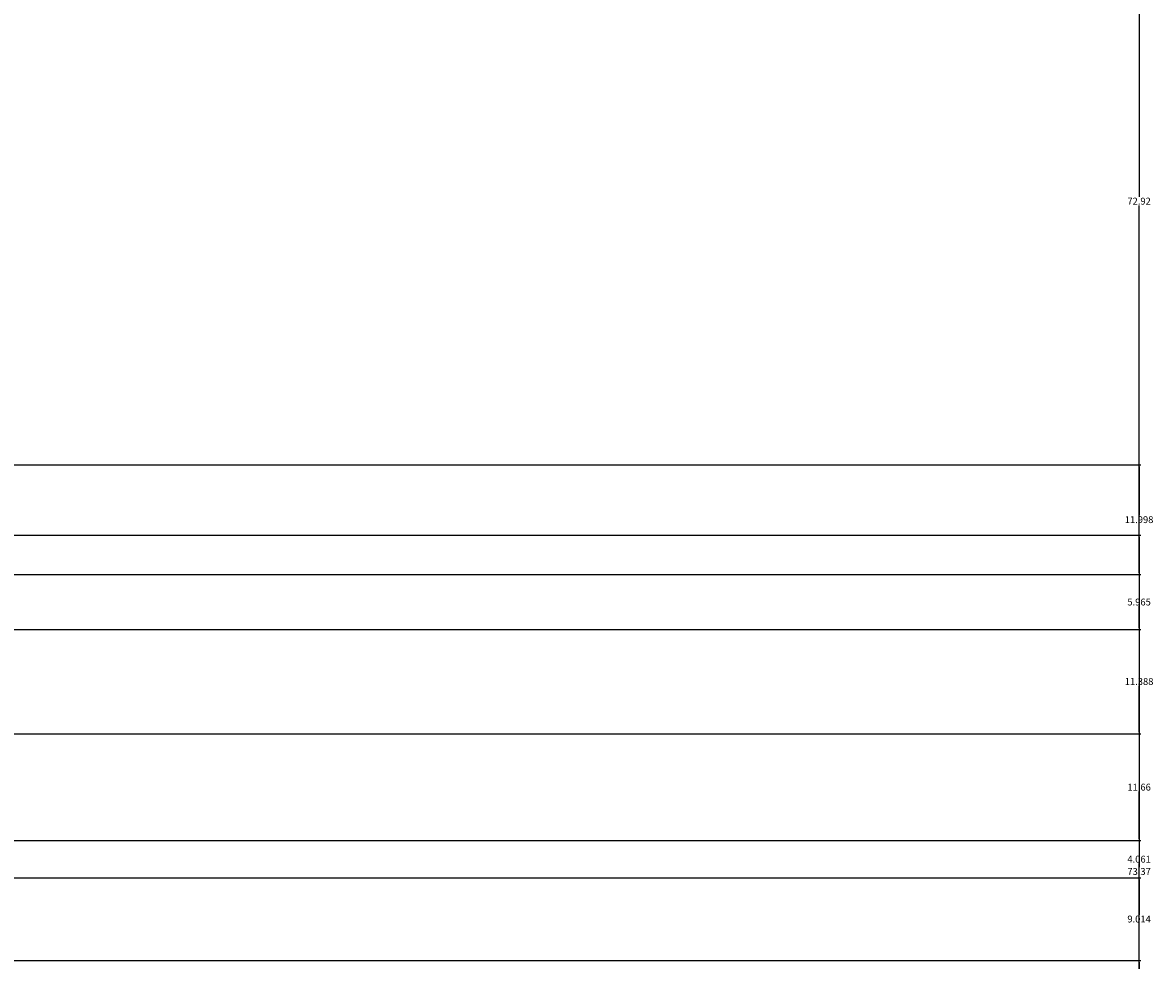
# Model space of a CAD drawing. Units: inches. Extents: x 62 to 566, y 66 to 528.
# Tile 19 of 20: x 443 to 566, y 298 to 401. Entities that reach past the tile are written whole.
import ezdxf

# ---------------------------------------------------------------- set-up
doc = ezdxf.new("R2010")
doc.units = ezdxf.units.IN
doc.header["$MEASUREMENT"] = 0
doc.layers.add('A-ANNO-DIMS', color=2, linetype='Continuous', lineweight=18)
doc.styles.get("Standard").update_dxf_attribs({"font": 'arial.ttf'})
doc.dimstyles.get("Standard").update_dxf_attribs({"dimtxt": 0.75, "dimasz": 0.18, "dimexe": 0.18, "dimexo": 0.0625, "dimgap": 0.09, "dimtad": 0, "dimtih": 1, "dimtoh": 1, "dimdec": 4, "dimzin": 0, "dimdsep": 46, "dimlunit": 4, "dimtxsty": 'Standard', "dimcen": 0.09, "dimadec": 0, "dimazin": 0, "dimtfac": 1, "dimtdec": 4, "dimtofl": 0, "dimtmove": 0, "dimatfit": 3, "dimfxl": 1, "dimtolj": 1, "dimtzin": 0, "dimarcsym": 0})

# ---------------------------------------------------------------- blocks, each defined once
blk = doc.blocks.new('*D23')
at = {"layer": 'A-ANNO-DIMS', "color": 0, "lineweight": -2, "transparency": 16777216}
for p, q in [((374.2, 344.78), (564.47, 344.78)), ((564.29, 344.6), (564.29, 308.57)), ((564.29, 271.59), (564.29, 307.62)), ((540.1, 271.41), (564.47, 271.41))]:
    blk.add_line(p, q, dxfattribs=at)
at = {"layer": 'A-ANNO-DIMS', "color": 0, "transparency": 16777216}
for points in [[(564.26, 344.6), (564.32, 344.6), (564.29, 344.78)], [(564.26, 271.59), (564.32, 271.59), (564.29, 271.41)]]:
    blk.add_solid(points, dxfattribs=at)
at = {"layer": 'Defpoints', "color": 0, "transparency": 16777216}
for p in [(374.14, 344.78), (564.29, 344.78), (540.04, 271.41)]:
    blk.add_point(p, dxfattribs=at)
at = {"layer": 'A-ANNO-DIMS', "color": 0, "transparency": 16777216, "insert": (564.29, 308.1), "char_height": 0.75, "attachment_point": 5}
blk.add_mtext('\\A1;73.37', dxfattribs=at)
blk = doc.blocks.new('*D24')
at = {"layer": 'A-ANNO-DIMS', "color": 0, "lineweight": -2, "transparency": 16777216}
for p, q in [((374.2, 417.71), (564.47, 417.71)), ((564.29, 417.53), (564.29, 381.72)), ((564.29, 344.96), (564.29, 380.77)), ((374.2, 344.78), (564.47, 344.78))]:
    blk.add_line(p, q, dxfattribs=at)
at = {"layer": 'A-ANNO-DIMS', "color": 0, "transparency": 16777216}
for points in [[(564.26, 417.53), (564.32, 417.53), (564.29, 417.71)], [(564.26, 344.96), (564.32, 344.96), (564.29, 344.78)]]:
    blk.add_solid(points, dxfattribs=at)
at = {"layer": 'Defpoints', "color": 0, "transparency": 16777216}
for p in [(374.14, 417.71), (564.29, 417.71), (374.14, 344.78)]:
    blk.add_point(p, dxfattribs=at)
at = {"layer": 'A-ANNO-DIMS', "color": 0, "transparency": 16777216, "insert": (564.29, 381.24), "char_height": 0.75, "attachment_point": 5}
blk.add_mtext('\\A1;72.92', dxfattribs=at)
blk = doc.blocks.new('*D91')
at = {"layer": 'A-ANNO-DIMS', "color": 0, "lineweight": -2, "transparency": 16777216}
for p, q in [((433.87, 298.4), (564.47, 298.4)), ((564.29, 298.22), (564.29, 297.15)), ((564.29, 295.13), (564.29, 296.2)), ((433.87, 294.95), (564.47, 294.95))]:
    blk.add_line(p, q, dxfattribs=at)
at = {"layer": 'A-ANNO-DIMS', "color": 0, "transparency": 16777216}
for points in [[(564.26, 298.22), (564.32, 298.22), (564.29, 298.4)], [(564.26, 295.13), (564.32, 295.13), (564.29, 294.95)]]:
    blk.add_solid(points, dxfattribs=at)
at = {"layer": 'Defpoints', "color": 0, "transparency": 16777216}
for p in [(433.81, 298.4), (564.29, 298.4), (433.81, 294.95)]:
    blk.add_point(p, dxfattribs=at)
at = {"layer": 'A-ANNO-DIMS', "color": 0, "transparency": 16777216, "insert": (564.29, 296.67), "char_height": 0.75, "attachment_point": 5}
blk.add_mtext('\\A1;3.449', dxfattribs=at)
blk = doc.blocks.new('*D92')
at = {"layer": 'A-ANNO-DIMS', "color": 0, "lineweight": -2, "transparency": 16777216}
for p, q in [((392.54, 307.41), (564.47, 307.41)), ((564.29, 307.23), (564.29, 303.38)), ((564.29, 298.58), (564.29, 302.43)), ((433.87, 298.4), (564.47, 298.4))]:
    blk.add_line(p, q, dxfattribs=at)
at = {"layer": 'A-ANNO-DIMS', "color": 0, "transparency": 16777216}
for points in [[(564.26, 307.23), (564.32, 307.23), (564.29, 307.41)], [(564.26, 298.58), (564.32, 298.58), (564.29, 298.4)]]:
    blk.add_solid(points, dxfattribs=at)
at = {"layer": 'Defpoints', "color": 0, "transparency": 16777216}
for p in [(392.48, 307.41), (564.29, 307.41), (433.81, 298.4)]:
    blk.add_point(p, dxfattribs=at)
at = {"layer": 'A-ANNO-DIMS', "color": 0, "transparency": 16777216, "insert": (564.29, 302.91), "char_height": 0.75, "attachment_point": 5}
blk.add_mtext('\\A1;9.014', dxfattribs=at)
blk = doc.blocks.new('*D93')
at = {"layer": 'A-ANNO-DIMS', "color": 0, "lineweight": -2, "transparency": 16777216}
for p, q in [((433.23, 311.47), (564.47, 311.47)), ((564.29, 311.29), (564.29, 309.92)), ((564.29, 307.59), (564.29, 308.97)), ((392.54, 307.41), (564.47, 307.41))]:
    blk.add_line(p, q, dxfattribs=at)
at = {"layer": 'A-ANNO-DIMS', "color": 0, "transparency": 16777216}
for points in [[(564.26, 311.29), (564.32, 311.29), (564.29, 311.47)], [(564.26, 307.59), (564.32, 307.59), (564.29, 307.41)]]:
    blk.add_solid(points, dxfattribs=at)
at = {"layer": 'Defpoints', "color": 0, "transparency": 16777216}
for p in [(433.16, 311.47), (564.29, 311.47), (392.48, 307.41)]:
    blk.add_point(p, dxfattribs=at)
at = {"layer": 'A-ANNO-DIMS', "color": 0, "transparency": 16777216, "insert": (564.29, 309.44), "char_height": 0.75, "attachment_point": 5}
blk.add_mtext('\\A1;4.061', dxfattribs=at)
blk = doc.blocks.new('*D94')
at = {"layer": 'A-ANNO-DIMS', "color": 0, "lineweight": -2, "transparency": 16777216}
for p, q in [((433.23, 323.13), (564.47, 323.13)), ((564.29, 322.95), (564.29, 317.78)), ((564.29, 311.65), (564.29, 316.83)), ((433.23, 311.47), (564.47, 311.47))]:
    blk.add_line(p, q, dxfattribs=at)
at = {"layer": 'A-ANNO-DIMS', "color": 0, "transparency": 16777216}
for points in [[(564.26, 322.95), (564.32, 322.95), (564.29, 323.13)], [(564.26, 311.65), (564.32, 311.65), (564.29, 311.47)]]:
    blk.add_solid(points, dxfattribs=at)
at = {"layer": 'Defpoints', "color": 0, "transparency": 16777216}
for p in [(433.16, 323.13), (564.29, 323.13), (433.16, 311.47)]:
    blk.add_point(p, dxfattribs=at)
at = {"layer": 'A-ANNO-DIMS', "color": 0, "transparency": 16777216, "insert": (564.29, 317.3), "char_height": 0.75, "attachment_point": 5}
blk.add_mtext('\\A1;11.66', dxfattribs=at)
blk = doc.blocks.new('*D95')
at = {"layer": 'A-ANNO-DIMS', "color": 0, "lineweight": -2, "transparency": 16777216}
for p, q in [((433.23, 334.52), (564.47, 334.52)), ((564.29, 334.34), (564.29, 329.3)), ((564.29, 323.31), (564.29, 328.35)), ((433.23, 323.13), (564.47, 323.13))]:
    blk.add_line(p, q, dxfattribs=at)
at = {"layer": 'A-ANNO-DIMS', "color": 0, "transparency": 16777216}
for points in [[(564.26, 334.34), (564.32, 334.34), (564.29, 334.52)], [(564.26, 323.31), (564.32, 323.31), (564.29, 323.13)]]:
    blk.add_solid(points, dxfattribs=at)
at = {"layer": 'Defpoints', "color": 0, "transparency": 16777216}
for p in [(433.16, 334.52), (564.29, 334.52), (433.16, 323.13)]:
    blk.add_point(p, dxfattribs=at)
at = {"layer": 'A-ANNO-DIMS', "color": 0, "transparency": 16777216, "insert": (564.29, 328.83), "char_height": 0.75, "attachment_point": 5}
blk.add_mtext('\\A1;11.388', dxfattribs=at)
blk = doc.blocks.new('*D96')
at = {"layer": 'A-ANNO-DIMS', "color": 0, "lineweight": -2, "transparency": 16777216}
for p, q in [((433.23, 340.49), (564.47, 340.49)), ((564.29, 340.31), (564.29, 337.98)), ((564.29, 334.7), (564.29, 337.03)), ((433.23, 334.52), (564.47, 334.52))]:
    blk.add_line(p, q, dxfattribs=at)
at = {"layer": 'A-ANNO-DIMS', "color": 0, "transparency": 16777216}
for points in [[(564.26, 340.31), (564.32, 340.31), (564.29, 340.49)], [(564.26, 334.7), (564.32, 334.7), (564.29, 334.52)]]:
    blk.add_solid(points, dxfattribs=at)
at = {"layer": 'Defpoints', "color": 0, "transparency": 16777216}
for p in [(433.16, 340.49), (564.29, 340.49), (433.16, 334.52)]:
    blk.add_point(p, dxfattribs=at)
at = {"layer": 'A-ANNO-DIMS', "color": 0, "transparency": 16777216, "insert": (564.29, 337.5), "char_height": 0.75, "attachment_point": 5}
blk.add_mtext('\\A1;5.965', dxfattribs=at)
blk = doc.blocks.new('*D97')
at = {"layer": 'A-ANNO-DIMS', "color": 0, "lineweight": -2, "transparency": 16777216}
for p, q in [((439.75, 352.48), (564.47, 352.48)), ((564.29, 352.3), (564.29, 346.96)), ((564.29, 340.67), (564.29, 346.01)), ((433.23, 340.49), (564.47, 340.49))]:
    blk.add_line(p, q, dxfattribs=at)
at = {"layer": 'A-ANNO-DIMS', "color": 0, "transparency": 16777216}
for points in [[(564.26, 352.3), (564.32, 352.3), (564.29, 352.48)], [(564.26, 340.67), (564.32, 340.67), (564.29, 340.49)]]:
    blk.add_solid(points, dxfattribs=at)
at = {"layer": 'Defpoints', "color": 0, "transparency": 16777216}
for p in [(439.69, 352.48), (564.29, 352.48), (433.16, 340.49)]:
    blk.add_point(p, dxfattribs=at)
at = {"layer": 'A-ANNO-DIMS', "color": 0, "transparency": 16777216, "insert": (564.29, 346.49), "char_height": 0.75, "attachment_point": 5}
blk.add_mtext('\\A1;11.998', dxfattribs=at)

msp = doc.modelspace()

# ---------------------------------------------------------------- dimensions: what is measured, and where the dimension line sits
at = {"layer": 'A-ANNO-DIMS'}
for base, p1, p2, override, picture, middle in [((564.2868, 417.7059), (374.1373, 344.7821), (374.1373, 417.7059), {"dimdec": 2, "dimlfac": 1, "dimrnd": 0, "dimzin": 0, "dimdsep": 46, "dimlunit": 2}, '*D24', (564.2868, 381.244)), ((564.28678, 352.4848), (433.16362, 340.48631), (439.68784, 352.4848), {"dimdec": 3, "dimlfac": 1, "dimrnd": 0, "dimzin": 0, "dimdsep": 46, "dimlunit": 2}, '*D97', (564.28678, 346.48556)), ((564.2868, 344.7821), (540.0368, 271.4128), (374.1373, 344.7821), {"dimdec": 2, "dimlfac": 1, "dimrnd": 0, "dimzin": 0, "dimdsep": 46, "dimlunit": 2}, '*D23', (564.2868, 308.0974)), ((564.2868, 340.4863), (433.1636, 334.5211), (433.1636, 340.4863), {"dimdec": 3, "dimlfac": 1, "dimrnd": 0, "dimzin": 0, "dimdsep": 46, "dimlunit": 2}, '*D96', (564.2868, 337.5037)), ((564.2868, 334.5211), (433.1636, 323.1329), (433.1636, 334.5211), {"dimdec": 3, "dimlfac": 1, "dimrnd": 0, "dimzin": 0, "dimdsep": 46, "dimlunit": 2}, '*D95', (564.2868, 328.827)), ((564.2868, 323.1329), (433.1636, 311.4736), (433.1636, 323.1329), {"dimdec": 2, "dimlfac": 1, "dimrnd": 0, "dimzin": 0, "dimdsep": 46, "dimlunit": 2}, '*D94', (564.2868, 317.3033)), ((564.2868, 311.4736), (392.4793, 307.4128), (433.1636, 311.4736), {"dimdec": 3, "dimlfac": 1, "dimrnd": 0, "dimzin": 0, "dimdsep": 46, "dimlunit": 2}, '*D93', (564.2868, 309.4432)), ((564.2868, 307.4128), (433.8102, 298.3985), (392.4793, 307.4128), {"dimdec": 3, "dimlfac": 1, "dimrnd": 0, "dimzin": 0, "dimdsep": 46, "dimlunit": 2}, '*D92', (564.2868, 302.9056)), ((564.2868, 298.3985), (433.8102, 294.9497), (433.8102, 298.3985), {"dimdec": 3, "dimlfac": 1, "dimrnd": 0, "dimzin": 0, "dimdsep": 46, "dimlunit": 2}, '*D91', (564.2868, 296.6741))]:
    dim = msp.add_linear_dim(base=base, p1=p1, p2=p2, angle=90, dimstyle='Standard', override=override, dxfattribs=at)
    dim.commit()
    dim.dimension.update_dxf_attribs({"geometry": picture, "text_midpoint": middle})

doc.saveas('drawing.dxf')
